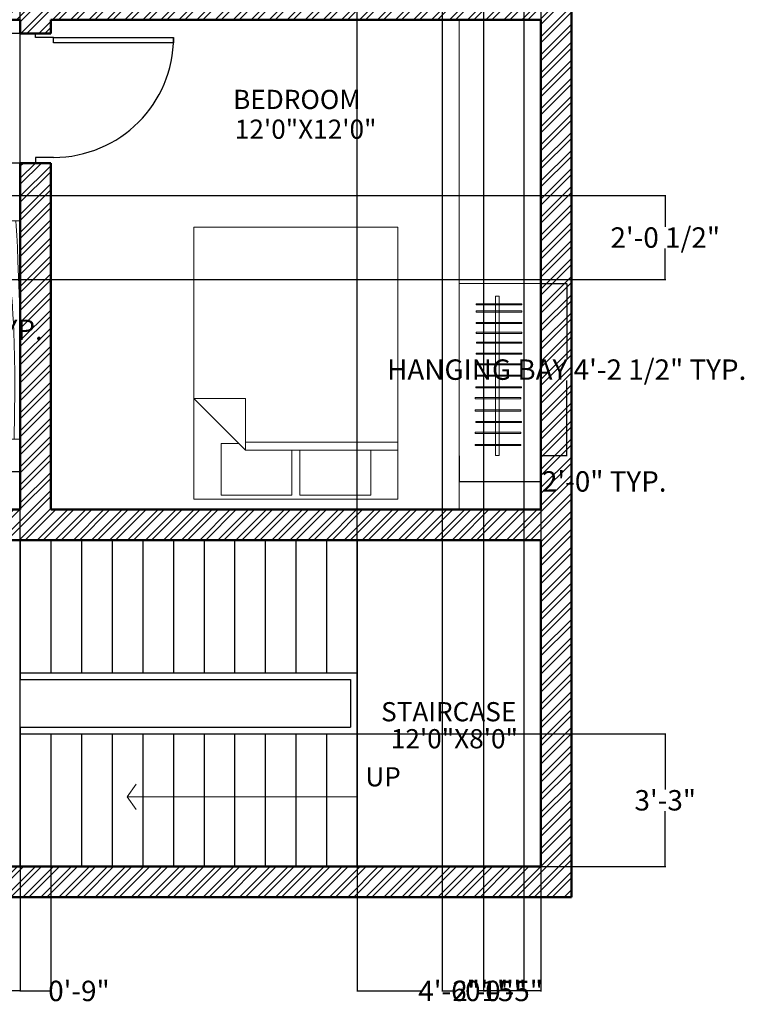
# Model space of a CAD drawing. Units: inches. Extents: x -71 to 434, y -519 to 67.
# Tile 3 of 7: x 221 to 434, y -514 to -224. Entities that reach past the tile are written whole.
import ezdxf

# ---------------------------------------------------------------- set-up
doc = ezdxf.new("R2010")
doc.units = ezdxf.units.IN
doc.header["$MEASUREMENT"] = 0
for name, color, linetype, lineweight in [('A-ANNO-DIMS', 7, 'Continuous', 18), ('A-ANNO-SYMB', 7, 'Continuous', 18), ('A-ANNO-TEXT', 7, 'Continuous', 25), ('A-AREA-IDEN', 7, 'Continuous', 25), ('A-FLOR-CASE', 9, 'Continuous', 18), ('A-WALL-PATT', 8, 'Continuous', 13), ('DOOR', 3, 'Continuous', 25), ('FURNITURE', 5, 'Continuous', 18), ('STAIR', 11, 'Continuous', 25), ('WALL', 50, 'Continuous', 50)]:
    doc.layers.add(name, color=color, linetype=linetype, lineweight=lineweight)
doc.styles.get("Standard").update_dxf_attribs({"font": 'arial.ttf'})
doc.dimstyles.get("Standard").update_dxf_attribs({"dimtxt": 6, "dimasz": 0.18, "dimexe": 0.18, "dimexo": 0.0625, "dimgap": 0.09, "dimtad": 0, "dimtih": 1, "dimtoh": 1, "dimdec": 0, "dimzin": 0, "dimdsep": 46, "dimlunit": 3, "dimtxsty": 'Standard', "dimcen": 0.09, "dimadec": 0, "dimazin": 0, "dimtfac": 1, "dimtdec": 0, "dimtofl": 0, "dimtmove": 0, "dimatfit": 3, "dimfxl": 1, "dimtolj": 1, "dimtzin": 0, "dimarcsym": 0})

# ---------------------------------------------------------------- blocks, each defined once
blk = doc.blocks.new('Bed - Queen')
for p, q in [((0, -80.00003), (0, 0)), ((0, 0), (59.99999, 0)), ((59.99999, 0), (59.99999, -80.00003)), ((7.99999, -1.2), (28.79998, -1.2)), ((7.99999, -14.4), (7.99999, -1.2)), ((28.79998, -1.2), (28.79998, -14.4)), ((31.19999, -1.2), (51.99999, -1.2)), ((31.19999, -14.4), (31.19999, -1.2)), ((51.99999, -1.2), (51.99999, -16.4)), ((0, -14.4), (44.8, -14.4)), ((59.99999, -29.6), (44.8, -14.4)), ((44.8, -14.4), (44.8, -29.6)), ((44.8, -16.8), (0, -16.8)), ((51.99999, -16.4), (46.79936, -16.4)), ((44.8, -29.6), (59.99999, -29.6)), ((59.99999, -80.00003), (0, -80.00003))]:
    blk.add_line(p, q)
blk = doc.blocks.new('*U13')
for p, q in [((0, 0), (0, -6)), ((40, 0), (40, -6))]:
    blk.add_line(p, q)
blk.add_lwpolyline([(0, 0), (0, 40), (1.75, 40), (1.75, 0)], close=True)
blk.add_arc((0, 0), 40, 0, 90)
blk = doc.blocks.new('Hutch - 19 x 72 in.')
for p, q in [((0, -19), (0, 0)), ((0, 0), (71.999994, 0)), ((71.999994, 0), (71.999994, -19)), ((71.999994, -19), (0, -19))]:
    blk.add_line(p, q)
for points in [[(26.99999, 0), (32.30411, -0.35238), (36.66731, -0.66276), (40.20336, -0.93603), (43.02603, -1.17708), (45.2491, -1.39079), (46.98632, -1.58203), (48.35147, -1.7557), (49.45833, -1.91667), (50.40388, -2.06917), (51.21809, -2.21484), (51.91414, -2.35465), (52.5052, -2.48958), (53.00447, -2.6206), (53.42512, -2.7487), (53.78035, -2.87484), (54.08333, -3), (54.34537, -3.12516), (54.57031, -3.2513), (54.76008, -3.37939), (54.91666, -3.51042), (55.04198, -3.64534), (55.13801, -3.78516), (55.2067, -3.93083), (55.24999, -4.08333), (55.26904, -4.24316), (55.26171, -4.40885), (55.22509, -4.57845), (55.15624, -4.75), (55.05224, -4.92155), (54.91015, -5.09115), (54.72704, -5.25684), (54.49999, -5.41667), (54.22493, -5.56934), (53.89322, -5.71615), (53.49511, -5.85905), (53.02083, -6), (52.4606, -6.14095), (51.80468, -6.28385), (51.04329, -6.43066), (50.16666, -6.58333), (49.16007, -6.74381), (47.98892, -6.91406), (46.61368, -7.09603), (44.99478, -7.29167), (43.09268, -7.50293), (40.86783, -7.73177), (38.28067, -7.98014), (35.29166, -8.25), (31.87654, -8.54053), (28.07226, -8.83984), (23.93107, -9.1333), (19.5052, -9.40625), (14.84692, -9.64404), (10.00846, -9.83203), (5.04207, -9.95557), (0, -10)], [(52.99999, 0), (54.87133, -0.53955), (56.39257, -1.03516), (57.61205, -1.48975), (58.57812, -1.90625), (59.3391, -2.2876), (59.94335, -2.63672), (60.4392, -2.95654), (60.87499, -3.25), (61.29247, -3.52002), (61.70702, -3.76953), (62.12743, -4.00146), (62.56249, -4.21875), (63.02099, -4.42432), (63.51171, -4.62109), (64.04345, -4.81201), (64.62499, -5), (65.26489, -5.1875), (65.9707, -5.375), (66.74975, -5.5625), (67.60937, -5.75), (68.55688, -5.9375), (69.5996, -6.125), (70.744867, -6.3125), (71.999994, -6.5)], [(61.49999, 0), (62.35961, -0.35254), (63.08007, -0.66406), (63.68627, -0.94043), (64.20312, -1.1875), (64.65551, -1.41113), (65.06835, -1.61719), (65.46655, -1.81152), (65.87499, -2), (66.31762, -2.1875), (66.81445, -2.375), (67.38452, -2.5625), (68.04687, -2.75), (68.82055, -2.9375), (69.7246, -3.125), (70.77807, -3.3125), (71.999994, -3.5)], [(0, -2), (11.2006, -2.34123), (19.90169, -2.62044), (26.43969, -2.84595), (31.15103, -3.02604), (34.37214, -3.16903), (36.43945, -3.2832), (37.68936, -3.37687), (38.45833, -3.45833), (39.02937, -3.53459), (39.472, -3.60742), (39.80232, -3.67733), (40.03645, -3.74479), (40.1905, -3.8103), (40.28059, -3.87435), (40.32283, -3.93742), (40.33333, -4), (40.32405, -4.0625), (40.29036, -4.125), (40.22346, -4.1875), (40.11458, -4.25), (39.95491, -4.3125), (39.73567, -4.375), (39.44807, -4.4375), (39.08333, -4.5), (38.62491, -4.56282), (38.02538, -4.6276), (37.22957, -4.69629), (36.18228, -4.77083), (34.82836, -4.85319), (33.11262, -4.94531), (30.97989, -5.04915), (28.37499, -5.16667), (25.27416, -5.29818), (21.77929, -5.4375), (18.02368, -5.57682), (14.14062, -5.70833), (10.26342, -5.82422), (6.52539, -5.91667), (3.05981, -5.97786), (0, -6)], [(71.999994, -9.5), (70.071934, -9.51147), (68.38801, -9.54492), (66.91113, -9.59888), (65.60416, -9.67187), (64.43001, -9.76245), (63.35156, -9.86914), (62.3317, -9.99048), (61.33333, -10.125), (60.32128, -10.27157), (59.26822, -10.43034), (58.14876, -10.60181), (56.93749, -10.78646), (55.60904, -10.98478), (54.13801, -11.19726), (52.49902, -11.4244), (50.66666, -11.66667), (48.62239, -11.92358), (46.37499, -12.19075), (43.9401, -12.46281), (41.33333, -12.73437), (38.57031, -13.00008), (35.66666, -13.25456), (32.63801, -13.49243), (29.49999, -13.70833), (26.26367, -13.89689), (22.92187, -14.05273), (19.46289, -14.17049), (15.875, -14.24479), (12.14648, -14.27026), (8.26562, -14.24154), (4.2207, -14.15324), (0, -14)], [(0, -17), (8.37556, -17.14274), (15.58268, -17.20443), (21.74194, -17.19775), (26.97395, -17.13542), (31.39933, -17.03011), (35.13866, -16.89453), (38.31257, -16.74137), (41.04166, -16.58333), (43.4322, -16.43083), (45.5332, -16.28516), (47.37931, -16.14534), (49.0052, -16.01042), (50.44555, -15.87939), (51.73502, -15.7513), (52.90828, -15.62516), (53.99999, -15.5), (55.04044, -15.37508), (56.04231, -15.25065), (57.01391, -15.1272), (57.96353, -15.00521), (58.89949, -14.88517), (59.83007, -14.76758), (60.76358, -14.65291), (61.70833, -14.54167), (62.6752, -14.43465), (63.68554, -14.33398), (64.76326, -14.24211), (65.93229, -14.16146), (67.21655, -14.09448), (68.63997, -14.04362), (70.226475, -14.01131), (71.999994, -14)], [(36.99999, -19), (42.40038, -18.8125), (47.95312, -18.625), (53.43554, -18.4375), (58.62499, -18.25), (63.29882, -18.0625), (67.23437, -17.875), (70.208978, -17.6875), (71.999994, -17.5)]]:
    blk.add_lwpolyline(points)
blk = doc.blocks.new('WARDROBE-HANGING-BAY')
blk.add_line((24, 50.57), (0, 50.57))
for points in [[(10.65, 46.88), (11.71, 46.88), (11.71, 0), (10.65, 0)], [(4.96, 44.68), (18.35, 44.68), (18.35, 44.35), (4.96, 44.35)], [(4.96, 42.56), (18.35, 42.56), (18.35, 42.22), (4.96, 42.22)], [(18.35, 38.84), (4.96, 38.84), (4.96, 39.17), (18.35, 39.17)], [(4.96, 36.28), (18.35, 36.28), (18.35, 35.95), (4.96, 35.95)], [(18.43, 33.04), (5.05, 33.04), (5.05, 33.37), (18.43, 33.37)], [(4.96, 30.15), (18.35, 30.15), (18.35, 29.82), (4.96, 29.82)], [(18.33, 26.66), (4.95, 26.66), (4.95, 26.99), (18.33, 26.99)], [(4.96, 23.69), (18.35, 23.69), (18.35, 23.36), (4.96, 23.36)], [(18.29, 19.89), (4.91, 19.89), (4.91, 20.22), (18.29, 20.22)], [(4.71, 17.05), (18.09, 17.05), (18.09, 16.72), (4.71, 16.72)], [(18.09, 13.11), (4.71, 13.11), (4.71, 13.44), (18.09, 13.44)], [(18.29, 9.72), (4.91, 9.72), (4.91, 10.05), (18.29, 10.05)], [(4.71, 6.88), (18.09, 6.88), (18.09, 6.55), (4.71, 6.55)], [(18.09, 2.94), (4.71, 2.94), (4.71, 3.27), (18.09, 3.27)]]:
    blk.add_lwpolyline(points, close=True)
blk = doc.blocks.new('*D32')
at = {"layer": 'A-ANNO-DIMS', "color": 0, "lineweight": -2, "transparency": 16777216}
for p, q in [((204.4, -283.25), (194.65, -283.25)), ((194.83, -283.43), (194.83, -312.16)), ((194.83, -347.28), (194.83, -318.55)), ((204.4, -347.46), (194.65, -347.46))]:
    blk.add_line(p, q, dxfattribs=at)
at = {"layer": 'A-ANNO-DIMS', "color": 0, "transparency": 16777216}
for points in [[(194.8, -283.43), (194.86, -283.43), (194.83, -283.25)], [(194.8, -347.28), (194.86, -347.28), (194.83, -347.46)]]:
    blk.add_solid(points, dxfattribs=at)
at = {"layer": 'Defpoints', "color": 0, "transparency": 16777216}
for p in [(194.83, -283.25), (204.46, -283.25), (204.46, -347.46)]:
    blk.add_point(p, dxfattribs=at)
at = {"layer": 'A-ANNO-DIMS', "color": 0, "transparency": 16777216, "insert": (194.83, -315.36), "char_height": 6, "attachment_point": 5}
blk.add_mtext('\\A1;HUTCH 5\'-4" TYP.', dxfattribs=at)
blk = doc.blocks.new('*D33')
at = {"layer": 'A-ANNO-DIMS', "color": 0, "lineweight": -2, "transparency": 16777216}
for p, q in [((204.46, -347.52), (204.46, -357.27)), ((221.41, -347.52), (221.41, -357.27)), ((204.46, -357.09), (204.28, -357.09)), ((221.23, -357.09), (204.64, -357.09))]:
    blk.add_line(p, q, dxfattribs=at)
at = {"layer": 'A-ANNO-DIMS', "color": 0, "transparency": 16777216}
for points in [[(204.64, -357.06), (204.64, -357.12), (204.46, -357.09)], [(221.23, -357.06), (221.23, -357.12), (221.41, -357.09)]]:
    blk.add_solid(points, dxfattribs=at)
at = {"layer": 'Defpoints', "color": 0, "transparency": 16777216}
for p in [(204.46, -347.46), (221.41, -347.46), (204.46, -357.09)]:
    blk.add_point(p, dxfattribs=at)
at = {"layer": 'A-ANNO-DIMS', "color": 0, "transparency": 16777216, "insert": (186.19, -357.09), "char_height": 6, "attachment_point": 5}
blk.add_mtext('\\A1;1\'-5" TYP.', dxfattribs=at)
blk = doc.blocks.new('*D38')
at = {"layer": 'A-ANNO-DIMS', "color": 0, "lineweight": -2, "transparency": 16777216}
for p, q in [((374.47, -301.76), (382.17, -301.76)), ((381.99, -301.94), (381.99, -323.86)), ((381.99, -352.16), (381.99, -330.24)), ((374.47, -352.34), (382.17, -352.34))]:
    blk.add_line(p, q, dxfattribs=at)
at = {"layer": 'A-ANNO-DIMS', "color": 0, "transparency": 16777216}
for points in [[(381.96, -301.94), (382.02, -301.94), (381.99, -301.76)], [(381.96, -352.16), (382.02, -352.16), (381.99, -352.34)]]:
    blk.add_solid(points, dxfattribs=at)
at = {"layer": 'Defpoints', "color": 0, "transparency": 16777216}
for p in [(374.41, -301.76), (381.99, -301.76), (374.41, -352.34)]:
    blk.add_point(p, dxfattribs=at)
at = {"layer": 'A-ANNO-DIMS', "color": 0, "transparency": 16777216, "insert": (381.99, -327.05), "char_height": 6, "attachment_point": 5}
blk.add_mtext('\\A1;HANGING BAY 4\'-2 1/2" TYP.', dxfattribs=at)
blk = doc.blocks.new('*D39')
at = {"layer": 'A-ANNO-DIMS', "color": 0, "lineweight": -2, "transparency": 16777216}
for p, q in [((350.41, -352.4), (350.41, -360.1)), ((374.41, -352.4), (374.41, -360.1)), ((350.59, -359.92), (374.23, -359.92)), ((374.41, -359.92), (374.59, -359.92))]:
    blk.add_line(p, q, dxfattribs=at)
at = {"layer": 'A-ANNO-DIMS', "color": 0, "transparency": 16777216}
for points in [[(350.59, -359.89), (350.59, -359.95), (350.41, -359.92)], [(374.23, -359.89), (374.23, -359.95), (374.41, -359.92)]]:
    blk.add_solid(points, dxfattribs=at)
at = {"layer": 'Defpoints', "color": 0, "transparency": 16777216}
for p in [(350.41, -352.34), (374.41, -352.34), (374.41, -359.92)]:
    blk.add_point(p, dxfattribs=at)
at = {"layer": 'A-ANNO-DIMS', "color": 0, "transparency": 16777216, "insert": (393.02, -359.92), "char_height": 6, "attachment_point": 5}
blk.add_mtext('\\A1;2\'-0" TYP.', dxfattribs=at)
blk = doc.blocks.new('*D49')
at = {"layer": 'A-ANNO-DIMS', "color": 0, "lineweight": -2, "transparency": 16777216}
for p, q in [((221.41, -473.1), (221.41, 58.56)), ((221.59, 58.38), (262.84, 58.38)), ((320.23, 58.38), (278.98, 58.38)), ((320.41, -473.1), (320.41, 58.56))]:
    blk.add_line(p, q, dxfattribs=at)
at = {"layer": 'A-ANNO-DIMS', "color": 0, "transparency": 16777216}
for points in [[(221.59, 58.41), (221.59, 58.35), (221.41, 58.38)], [(320.23, 58.41), (320.23, 58.35), (320.41, 58.38)]]:
    blk.add_solid(points, dxfattribs=at)
at = {"layer": 'Defpoints', "color": 0, "transparency": 16777216}
for p in [(320.41, 58.38), (221.41, -473.17), (320.41, -473.17)]:
    blk.add_point(p, dxfattribs=at)
at = {"layer": 'A-ANNO-DIMS', "color": 0, "transparency": 16777216, "insert": (270.91, 58.38), "char_height": 6, "attachment_point": 5}
blk.add_mtext('\\A1;8\'-3"', dxfattribs=at)
blk = doc.blocks.new('*D50')
at = {"layer": 'A-ANNO-DIMS', "color": 0, "lineweight": -2, "transparency": 16777216}
for p, q in [((320.41, -473.23), (320.41, -509.9)), ((374.41, -473.23), (374.41, -509.9)), ((320.59, -509.72), (339.22, -509.72)), ((374.23, -509.72), (355.59, -509.72))]:
    blk.add_line(p, q, dxfattribs=at)
at = {"layer": 'A-ANNO-DIMS', "color": 0, "transparency": 16777216}
for points in [[(320.59, -509.69), (320.59, -509.75), (320.41, -509.72)], [(374.23, -509.69), (374.23, -509.75), (374.41, -509.72)]]:
    blk.add_solid(points, dxfattribs=at)
at = {"layer": 'Defpoints', "color": 0, "transparency": 16777216}
for p in [(320.41, -473.17), (374.41, -473.17), (374.41, -509.72)]:
    blk.add_point(p, dxfattribs=at)
at = {"layer": 'A-ANNO-DIMS', "color": 0, "transparency": 16777216, "insert": (347.41, -509.72), "char_height": 6, "attachment_point": 5}
blk.add_mtext('\\A1;4\'-6"', dxfattribs=at)
blk = doc.blocks.new('*D51')
at = {"layer": 'A-ANNO-DIMS', "color": 0, "lineweight": -2, "transparency": 16777216}
for p, q in [((221.47, -434.17), (411.14, -434.17)), ((410.96, -434.35), (410.96, -450.51)), ((410.96, -472.99), (410.96, -456.82)), ((221.47, -473.17), (411.14, -473.17))]:
    blk.add_line(p, q, dxfattribs=at)
at = {"layer": 'A-ANNO-DIMS', "color": 0, "transparency": 16777216}
for points in [[(410.93, -434.35), (410.99, -434.35), (410.96, -434.17)], [(410.93, -472.99), (410.99, -472.99), (410.96, -473.17)]]:
    blk.add_solid(points, dxfattribs=at)
at = {"layer": 'Defpoints', "color": 0, "transparency": 16777216}
for p in [(221.41, -434.17), (410.96, -434.17), (221.41, -473.17)]:
    blk.add_point(p, dxfattribs=at)
at = {"layer": 'A-ANNO-DIMS', "color": 0, "transparency": 16777216, "insert": (410.96, -453.67), "char_height": 6, "attachment_point": 5}
blk.add_mtext('\\A1;3\'-3"', dxfattribs=at)
blk = doc.blocks.new('*D52')
at = {"layer": 'A-ANNO-DIMS', "color": 0, "lineweight": -2, "transparency": 16777216}
for p, q in [((221.41, -473.23), (221.41, -509.9)), ((230.41, -473.23), (230.41, -509.9)), ((221.59, -509.72), (230.23, -509.72)), ((230.41, -509.72), (230.59, -509.72))]:
    blk.add_line(p, q, dxfattribs=at)
at = {"layer": 'A-ANNO-DIMS', "color": 0, "transparency": 16777216}
for points in [[(221.59, -509.69), (221.59, -509.75), (221.41, -509.72)], [(230.23, -509.69), (230.23, -509.75), (230.41, -509.72)]]:
    blk.add_solid(points, dxfattribs=at)
at = {"layer": 'Defpoints', "color": 0, "transparency": 16777216}
for p in [(221.41, -473.17), (230.41, -473.17), (230.41, -509.72)]:
    blk.add_point(p, dxfattribs=at)
at = {"layer": 'A-ANNO-DIMS', "color": 0, "transparency": 16777216, "insert": (238.65, -509.72), "char_height": 6, "attachment_point": 5}
blk.add_mtext('\\A1;0\'-9"', dxfattribs=at)
blk = doc.blocks.new('*D54')
at = {"layer": 'A-ANNO-DIMS', "color": 0, "lineweight": -2, "transparency": 16777216}
for p, q in [((-3.59, -473.23), (-3.59, -509.9)), ((221.41, -473.23), (221.41, -509.9)), ((-3.41, -509.72), (98.79, -509.72)), ((221.23, -509.72), (119.02, -509.72))]:
    blk.add_line(p, q, dxfattribs=at)
at = {"layer": 'A-ANNO-DIMS', "color": 0, "transparency": 16777216}
for points in [[(-3.41, -509.69), (-3.41, -509.75), (-3.59, -509.72)], [(221.23, -509.69), (221.23, -509.75), (221.41, -509.72)]]:
    blk.add_solid(points, dxfattribs=at)
at = {"layer": 'Defpoints', "color": 0, "transparency": 16777216}
for p in [(-3.59, -473.17), (221.41, -473.17), (221.41, -509.72)]:
    blk.add_point(p, dxfattribs=at)
at = {"layer": 'A-ANNO-DIMS', "color": 0, "transparency": 16777216, "insert": (108.91, -509.72), "char_height": 6, "attachment_point": 5}
blk.add_mtext('\\A1;18\'-9"', dxfattribs=at)
blk = doc.blocks.new('*D55')
at = {"layer": 'A-ANNO-DIMS', "color": 0, "lineweight": -2, "transparency": 16777216}
for p, q in [((345.41, -119.23), (345.41, -509.9)), ((369.41, -119.23), (369.41, -509.9)), ((345.59, -509.72), (349.29, -509.72)), ((369.23, -509.72), (365.52, -509.72))]:
    blk.add_line(p, q, dxfattribs=at)
at = {"layer": 'A-ANNO-DIMS', "color": 0, "transparency": 16777216}
for points in [[(345.59, -509.69), (345.59, -509.75), (345.41, -509.72)], [(369.23, -509.69), (369.23, -509.75), (369.41, -509.72)]]:
    blk.add_solid(points, dxfattribs=at)
at = {"layer": 'Defpoints', "color": 0, "transparency": 16777216}
for p in [(345.41, -119.17), (369.41, -119.17), (369.41, -509.72)]:
    blk.add_point(p, dxfattribs=at)
at = {"layer": 'A-ANNO-DIMS', "color": 0, "transparency": 16777216, "insert": (357.41, -509.72), "char_height": 6, "attachment_point": 5}
blk.add_mtext('\\A1;2\'-0"', dxfattribs=at)
blk = doc.blocks.new('*D58')
at = {"layer": 'A-ANNO-DIMS', "color": 0, "lineweight": -2, "transparency": 16777216}
for p, q in [((221.35, -228.23), (-40.32, -228.23)), ((-40.14, -228.41), (-40.14, -244.13)), ((-40.14, -266.16), (-40.14, -250.44)), ((221.35, -266.34), (-40.32, -266.34))]:
    blk.add_line(p, q, dxfattribs=at)
at = {"layer": 'A-ANNO-DIMS', "color": 0, "transparency": 16777216}
for points in [[(-40.17, -228.41), (-40.11, -228.41), (-40.14, -228.23)], [(-40.17, -266.16), (-40.11, -266.16), (-40.14, -266.34)]]:
    blk.add_solid(points, dxfattribs=at)
at = {"layer": 'Defpoints', "color": 0, "transparency": 16777216}
for p in [(221.41, -228.23), (-40.14, -266.34), (221.41, -266.34)]:
    blk.add_point(p, dxfattribs=at)
at = {"layer": 'A-ANNO-DIMS', "color": 0, "transparency": 16777216, "insert": (-40.14, -247.29), "char_height": 6, "attachment_point": 5}
blk.add_mtext('\\A1;3\'-2"', dxfattribs=at)
blk = doc.blocks.new('*D63')
at = {"layer": 'A-ANNO-DIMS', "color": 0, "lineweight": -2, "transparency": 16777216}
for p, q in [((369.41, -119.23), (369.41, -509.9)), ((374.41, -119.23), (374.41, -509.9)), ((369.41, -509.72), (369.23, -509.72)), ((374.23, -509.72), (369.59, -509.72))]:
    blk.add_line(p, q, dxfattribs=at)
at = {"layer": 'A-ANNO-DIMS', "color": 0, "transparency": 16777216}
for points in [[(369.59, -509.69), (369.59, -509.75), (369.41, -509.72)], [(374.23, -509.69), (374.23, -509.75), (374.41, -509.72)]]:
    blk.add_solid(points, dxfattribs=at)
at = {"layer": 'Defpoints', "color": 0, "transparency": 16777216}
for p in [(369.41, -119.17), (374.41, -119.17), (369.41, -509.72)]:
    blk.add_point(p, dxfattribs=at)
at = {"layer": 'A-ANNO-DIMS', "color": 0, "transparency": 16777216, "insert": (361.16, -509.72), "char_height": 6, "attachment_point": 5}
blk.add_mtext('\\A1;0\'-5"', dxfattribs=at)
blk = doc.blocks.new('*D65')
at = {"layer": 'A-ANNO-DIMS', "color": 0, "lineweight": -2, "transparency": 16777216}
for p, q in [((357.54, -214.92), (357.54, -509.9)), ((374.41, -215.23), (374.41, -509.9)), ((357.72, -509.72), (358.19, -509.72)), ((374.23, -509.72), (373.76, -509.72))]:
    blk.add_line(p, q, dxfattribs=at)
at = {"layer": 'A-ANNO-DIMS', "color": 0, "transparency": 16777216}
for points in [[(357.72, -509.69), (357.72, -509.75), (357.54, -509.72)], [(374.23, -509.69), (374.23, -509.75), (374.41, -509.72)]]:
    blk.add_solid(points, dxfattribs=at)
at = {"layer": 'Defpoints', "color": 0, "transparency": 16777216}
for p in [(357.54, -214.86), (374.41, -215.17), (374.41, -509.72)]:
    blk.add_point(p, dxfattribs=at)
at = {"layer": 'A-ANNO-DIMS', "color": 0, "transparency": 16777216, "insert": (365.97, -509.72), "char_height": 6, "attachment_point": 5}
blk.add_mtext('\\A1;1\'-5"', dxfattribs=at)
blk = doc.blocks.new('*D72')
at = {"layer": 'A-ANNO-DIMS', "color": 0, "lineweight": -2, "transparency": 16777216}
for p, q in [((111.22, -275.87), (411.14, -275.87)), ((410.96, -276.05), (410.96, -285.03)), ((410.96, -300.39), (410.96, -291.41)), ((111.22, -300.57), (411.14, -300.57))]:
    blk.add_line(p, q, dxfattribs=at)
at = {"layer": 'A-ANNO-DIMS', "color": 0, "transparency": 16777216}
for points in [[(410.93, -276.05), (410.99, -276.05), (410.96, -275.87)], [(410.93, -300.39), (410.99, -300.39), (410.96, -300.57)]]:
    blk.add_solid(points, dxfattribs=at)
at = {"layer": 'Defpoints', "color": 0, "transparency": 16777216}
for p in [(111.15, -275.87), (111.15, -300.57), (410.96, -300.57)]:
    blk.add_point(p, dxfattribs=at)
at = {"layer": 'A-ANNO-DIMS', "color": 0, "transparency": 16777216, "insert": (410.96, -288.22), "char_height": 6, "attachment_point": 5}
blk.add_mtext('\\A1;2\'-0 1/2"', dxfattribs=at)

msp = doc.modelspace()

# ---------------------------------------------------------------- hatches: boundary and pattern name
at = {"layer": 'A-WALL-PATT'}
h = msp.add_hatch(dxfattribs=at)
h.set_pattern_fill('ANSI32', color=256, scale=10)
h.set_pattern_definition([(45, (-213.138, 0), (-2.65165, 2.65165), []), (45, (-211.37, 0), (-2.65165, 2.65165), [])])
h.paths.add_polyline_path([(383.41, 30.83), (230.41, 30.83), (149.41, 30.83), (-12.59, 30.83), (-12.59, -20.17), (-3.59, -20.17), (-3.59, 21.83), (140.41, 21.83), (140.41, 15.83), (149.41, 15.83), (149.41, 21.83), (221.41, 21.83), (221.41, 15.83), (230.41, 15.83), (230.41, 21.83), (374.41, 21.83), (374.41, -110.17), (369.41, -110.17), (369.41, -119.17), (374.41, -119.17), (374.41, -215.17), (320.41, -215.17), (320.41, -119.17), (345.41, -119.17), (345.41, -110.17), (221.41, -110.17), (221.41, -119.17), (311.41, -119.17), (311.41, -215.17), (192.42, -215.17), (192.42, -224.17), (221.41, -224.17), (221.41, -228.23), (230.41, -228.23), (230.41, -224.17), (374.41, -224.17), (374.41, -368.17), (230.41, -368.17), (230.41, -266.34), (221.41, -266.34), (221.41, -368.17), (192.08, -368.17), (192.08, -377.17), (230.41, -377.17), (374.41, -377.17), (374.41, -473.17), (230.41, -473.17), (212.41, -473.17), (212.41, -482.17), (383.41, -482.17), (383.41, -377.17), (383.41, -224.17), (383.41, -119.17)])
h.paths.add_polyline_path([(149.41, -110.17), (-3.59, -110.17), (-3.59, -68.17), (-12.59, -68.17), (-12.59, -276.67), (-3.59, -276.67), (-3.59, -224.17), (154.41, -224.17), (154.41, -215.17), (149.41, -215.17), (149.41, -154.17), (140.41, -154.17), (140.41, -215.17), (-3.59, -215.17), (-3.59, -119.17), (19.82, -119.17), (140.41, -119.17), (140.41, -124.17), (149.41, -124.17)])
h.paths.add_polyline_path([(84.91, -368.17), (-3.59, -368.17), (-3.59, -324.67), (-12.59, -324.67), (-12.59, -377.17), (-12.59, -401.17), (-3.59, -401.17), (-3.59, -377.17), (84.91, -377.17)], flags=17)
h.paths.add_polyline_path([(1.41, -473.17), (-3.59, -473.17), (-3.59, -468.17), (-12.59, -468.17), (-12.59, -482.17), (1.41, -482.17)], flags=17)

# ---------------------------------------------------------------- linework, layer by layer
at = {"layer": 'A-ANNO-SYMB'}
for q in [(255.5, -448.91), (255.5, -456.42), (320.41, -452.67)]:
    msp.add_line((252.79, -452.67), q, dxfattribs=at)
at = {"layer": 'A-FLOR-CASE'}
msp.add_line((350.41, -368.17), (350.41, -224.52), dxfattribs=at)
at = {"layer": 'DOOR'}
for p, q in [((225.91, -229.39), (225.91, -228.23)), ((225.91, -264.65), (225.91, -266.34))]:
    msp.add_line(p, q, dxfattribs=at)
at = {"layer": 'STAIR'}
for p, q in [((221.41, -377.17), (221.41, -418.17)), ((230.41, -377.17), (230.41, -416.17)), ((239.41, -377.17), (239.41, -416.17)), ((248.41, -377.17), (248.41, -416.17)), ((257.41, -377.17), (257.41, -416.17)), ((266.41, -377.17), (266.41, -416.17)), ((275.41, -377.17), (275.41, -416.17)), ((284.41, -377.17), (284.41, -416.17)), ((293.41, -377.17), (293.41, -416.17)), ((302.41, -377.17), (302.41, -416.17)), ((311.41, -377.17), (311.41, -416.17)), ((320.41, -377.17), (320.41, -473.17)), ((221.41, -416.17), (320.41, -416.17)), ((221.41, -418.17), (318.41, -418.17)), ((318.41, -418.17), (318.41, -432.17)), ((221.41, -432.17), (221.41, -473.17)), ((221.41, -432.17), (318.41, -432.17)), ((221.41, -434.17), (320.41, -434.17)), ((230.41, -434.17), (230.41, -473.17)), ((239.41, -434.17), (239.41, -473.17)), ((248.41, -434.17), (248.41, -473.17)), ((257.41, -434.17), (257.41, -473.17)), ((266.41, -434.17), (266.41, -473.17)), ((275.41, -434.17), (275.41, -473.17)), ((284.41, -434.17), (284.41, -473.17)), ((293.41, -434.17), (293.41, -473.17)), ((302.41, -434.17), (302.41, -473.17)), ((311.41, -434.17), (311.41, -473.17))]:
    msp.add_line(p, q, dxfattribs=at)
at = {"layer": 'WALL'}
for p, q in [((383.41, -119.17), (383.41, -224.17)), ((192.42, -224.17), (221.41, -224.17)), ((221.41, -224.17), (221.41, -228.23)), ((230.41, -224.17), (230.41, -228.23)), ((230.41, -224.17), (374.41, -224.17)), ((374.41, -224.17), (374.41, -368.17)), ((383.41, -224.17), (383.41, -377.17)), ((221.41, -228.23), (230.41, -228.23)), ((221.41, -266.34), (230.41, -266.34)), ((221.41, -266.34), (221.41, -368.17)), ((230.41, -266.34), (230.41, -368.17)), ((192.08, -368.17), (221.41, -368.17)), ((230.41, -368.17), (374.41, -368.17)), ((192.08, -377.17), (230.41, -377.17)), ((230.41, -377.17), (374.41, -377.17)), ((374.41, -377.17), (374.41, -473.17)), ((383.41, -377.17), (383.41, -482.17)), ((-3.59, -473.17), (230.41, -473.17)), ((230.41, -473.17), (374.41, -473.17)), ((-12.59, -482.17), (383.41, -482.17))]:
    msp.add_line(p, q, dxfattribs=at)

# ---------------------------------------------------------------- block references
at = {"layer": 'A-FLOR-CASE'}
msp.add_blockref('WARDROBE-HANGING-BAY', (350.41, -352.34), dxfattribs=at)
at = {"layer": 'DOOR', "xscale": 0.88145672357558, "yscale": 0.88145672357558, "zscale": 0.88145672357558, "rotation": 270}
msp.add_blockref('*U13', (231.2, -229.39), dxfattribs=at)
at = {"layer": 'FURNITURE', "xscale": 0.8917373781469976, "yscale": 0.8917373781469976, "zscale": 0.8917373781469976, "rotation": 90}
msp.add_blockref('Hutch - 19 x 72 in.', (204.46, -347.46), dxfattribs=at)
at = {"layer": 'FURNITURE', "rotation": 180}
msp.add_blockref('Bed - Queen', (332.41, -365.13), dxfattribs=at)

# ---------------------------------------------------------------- texts
at = {"layer": 'A-ANNO-TEXT'}
msp.add_text('UP', height=5.643, dxfattribs=at).set_placement((322.81, -449.58))
at = {"layer": 'A-AREA-IDEN'}
for s, height, p in [('BEDROOM', 5.643, (283.96, -250.43)), ('12\'0"X12\'0"', 5.6432, (284.46, -259.19)), ('STAIRCASE', 5.643, (327.44, -430.45)), ('12\'0"X8\'0"', 5.643, (330.31, -438.39))]:
    msp.add_text(s, height=height, dxfattribs=at).set_placement(p)

# ---------------------------------------------------------------- dimensions: what is measured, and where the dimension line sits
at = {"layer": 'A-ANNO-DIMS'}
for base, p1, p2, picture, middle in [((320.41, 58.38), (221.41, -473.17), (320.41, -473.17), '*D49', (270.91, 58.38)), ((369.41, -509.72), (345.41, -119.17), (369.41, -119.17), '*D55', (357.41, -509.72)), ((369.41, -509.72), (374.41, -119.17), (369.41, -119.17), '*D63', (361.16, -509.72)), ((374.41, -509.72), (357.54, -214.86), (374.41, -215.17), '*D65', (365.97, -509.72)), ((221.41, -509.72), (-3.59, -473.17), (221.41, -473.17), '*D54', (108.91, -509.72)), ((230.41, -509.72), (221.41, -473.17), (230.41, -473.17), '*D52', (238.65, -509.72)), ((374.41, -509.72), (320.41, -473.17), (374.41, -473.17), '*D50', (347.41, -509.72))]:
    dim = msp.add_linear_dim(base=base, p1=p1, p2=p2, dimstyle='Standard', override={"dimdec": 1, "dimlfac": 1, "dimrnd": 0, "dimzin": 1, "dimdsep": 46, "dimlunit": 4, "dimfrac": 2}, dxfattribs=at)
    dim.commit()
    dim.dimension.update_dxf_attribs({"geometry": picture, "text_midpoint": middle})
for base, p1, p2, picture, middle in [((-40.14, -266.34), (221.41, -228.23), (221.41, -266.34), '*D58', (-40.14, -247.29)), ((410.96, -300.57), (111.15, -275.87), (111.15, -300.57), '*D72', (410.96, -288.22)), ((410.96, -434.17), (221.41, -473.17), (221.41, -434.17), '*D51', (410.96, -453.67))]:
    dim = msp.add_linear_dim(base=base, p1=p1, p2=p2, angle=90, dimstyle='Standard', override={"dimdec": 1, "dimlfac": 1, "dimrnd": 0, "dimzin": 1, "dimdsep": 46, "dimlunit": 4, "dimfrac": 2}, dxfattribs=at)
    dim.commit()
    dim.dimension.update_dxf_attribs({"geometry": picture, "text_midpoint": middle})
for base, p1, p2, angle, text, picture, middle in [((194.83, -283.25), (204.46, -347.46), (204.46, -283.25), 90, 'HUTCH <> TYP.', '*D32', (194.83, -315.36)), ((381.99, -301.76), (374.41, -352.34), (374.41, -301.76), 90, 'HANGING BAY <> TYP.', '*D38', (381.99, -327.05)), ((204.4648, -357.0885), (221.4078, -347.4577), (204.4648, -347.4577), 180, '<> TYP.', '*D33', (186.1907, -357.0885))]:
    dim = msp.add_linear_dim(base=base, p1=p1, p2=p2, angle=angle, text=text, dimstyle='Standard', override={"dimdec": 1, "dimlfac": 1, "dimrnd": 0, "dimzin": 1, "dimdsep": 46, "dimlunit": 4, "dimfrac": 2}, dxfattribs=at)
    dim.commit()
    dim.dimension.update_dxf_attribs({"geometry": picture, "text_midpoint": middle})
dim = msp.add_linear_dim(base=(374.41, -359.92), p1=(350.41, -352.34), p2=(374.41, -352.34), text='<> TYP.', dimstyle='Standard', override={"dimdec": 1, "dimlfac": 1, "dimrnd": 0, "dimzin": 1, "dimdsep": 46, "dimlunit": 4, "dimfrac": 2}, dxfattribs=at)
dim.commit()
dim.dimension.update_dxf_attribs({"geometry": '*D39', "text_midpoint": (393.02, -359.92)})

doc.saveas('drawing.dxf')
